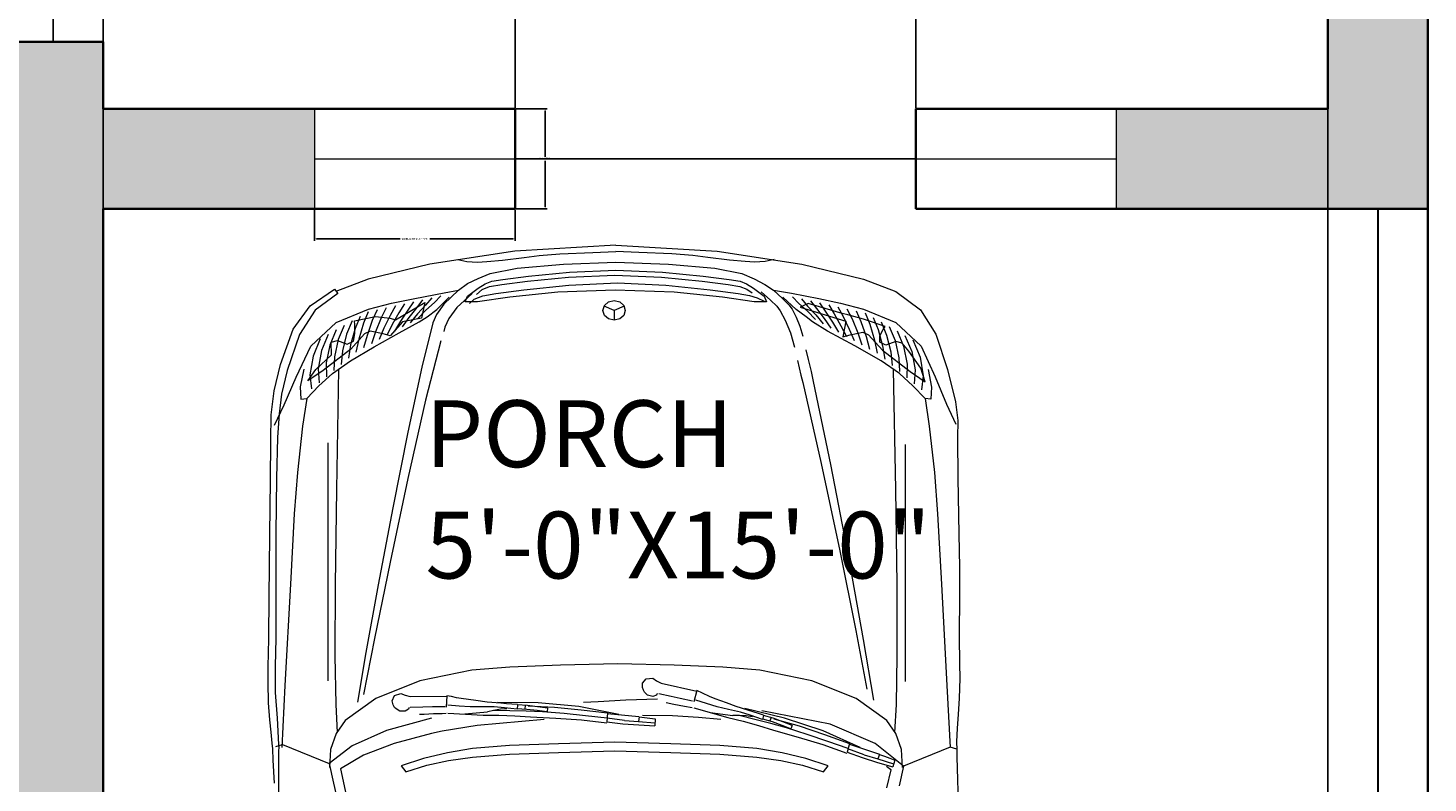
# Model space of a CAD drawing. Units: inches. Extents: x -16 to 587, y -783 to 64.
# Tile 6 of 14: x 111 to 237, y -595 to -527. Entities that reach past the tile are written whole.
import ezdxf

# ---------------------------------------------------------------- set-up
doc = ezdxf.new("R2010")
doc.units = ezdxf.units.IN
doc.header["$MEASUREMENT"] = 0
for name, color, linetype, lineweight in [('A-ANNO-DIMS', 2, 'Continuous', 18), ('A-AREA-IDEN', 7, 'Continuous', 18), ('A-DOOR', 3, 'Continuous', 25), ('A-GLAZ', 4, 'Continuous', 18), ('A-SITE-VEHC', 8, 'Continuous', 13), ('A-SITE-WALL', 7, 'Continuous', 30), ('A-WALL', 7, 'Continuous', 35), ('A-WALL-PATT', 23, 'Continuous', 13)]:
    doc.layers.add(name, color=color, linetype=linetype, lineweight=lineweight)
doc.styles.get("Standard").update_dxf_attribs({"font": 'arial.ttf'})
doc.dimstyles.get("Standard").update_dxf_attribs({"dimtxt": 0.18, "dimasz": 0.18, "dimexe": 0.18, "dimexo": 0.0625, "dimgap": 0.09, "dimtad": 0, "dimtih": 1, "dimtoh": 1, "dimdec": 0, "dimzin": 0, "dimdsep": 46, "dimlunit": 3, "dimtxsty": 'Standard', "dimcen": 0.09, "dimadec": 0, "dimazin": 0, "dimtfac": 1, "dimtdec": 0, "dimtofl": 0, "dimtmove": 0, "dimatfit": 3, "dimfxl": 1, "dimtolj": 1, "dimtzin": 0, "dimarcsym": 0})

# ---------------------------------------------------------------- blocks, each defined once
blk = doc.blocks.new('WIN-18-SIDELIGHT')
for p, q in [((6, 9), (0, 9)), ((0, 9), (0, 0)), ((6, 9), (18, 9)), ((18, 9), (18, 0)), ((0, 4.5), (18, 4.5)), ((0, 0), (6, 0)), ((18, 0), (6, 0))]:
    blk.add_line(p, q)
blk = doc.blocks.new('*D48')
at = {"layer": 'A-ANNO-DIMS', "color": 0, "lineweight": -2, "transparency": 16777216}
for p, q in [((137.08, -543.62), (137.08, -546.43)), ((155.08, -543.62), (155.08, -546.43)), ((137.26, -546.25), (144.75, -546.25)), ((154.9, -546.25), (147.42, -546.25))]:
    blk.add_line(p, q, dxfattribs=at)
at = {"layer": 'A-ANNO-DIMS', "color": 0, "transparency": 16777216}
for points in [[(137.26, -546.22), (137.26, -546.28), (137.08, -546.25)], [(154.9, -546.22), (154.9, -546.28), (155.08, -546.25)]]:
    blk.add_solid(points, dxfattribs=at)
at = {"layer": 'Defpoints', "color": 0, "transparency": 16777216}
for p in [(137.08, -543.55), (155.08, -543.55), (155.08, -546.25)]:
    blk.add_point(p, dxfattribs=at)
at = {"layer": 'A-ANNO-DIMS', "color": 0, "transparency": 16777216, "insert": (146.08, -546.25), "char_height": 0.18, "attachment_point": 5}
blk.add_mtext('\\A1;SIDELIGHT 1\'-6" TYP.', dxfattribs=at)
blk = doc.blocks.new('*D49')
at = {"layer": 'A-ANNO-DIMS', "color": 0, "lineweight": -2, "transparency": 16777216}
for p, q in [((155.15, -534.55), (157.96, -534.55)), ((157.78, -534.73), (157.78, -538.87)), ((157.78, -543.37), (157.78, -539.24)), ((155.15, -543.55), (157.96, -543.55))]:
    blk.add_line(p, q, dxfattribs=at)
at = {"layer": 'A-ANNO-DIMS', "color": 0, "transparency": 16777216}
for points in [[(157.75, -534.73), (157.81, -534.73), (157.78, -534.55)], [(157.75, -543.37), (157.81, -543.37), (157.78, -543.55)]]:
    blk.add_solid(points, dxfattribs=at)
at = {"layer": 'Defpoints', "color": 0, "transparency": 16777216}
for p in [(155.08, -534.55), (157.78, -534.55), (155.08, -543.55)]:
    blk.add_point(p, dxfattribs=at)
at = {"layer": 'A-ANNO-DIMS', "color": 0, "transparency": 16777216, "insert": (157.78, -539.05), "char_height": 0.18, "attachment_point": 5}
blk.add_mtext('\\A1;0\'-9" TYP.', dxfattribs=at)
blk = doc.blocks.new('*D56')
at = {"layer": 'A-ANNO-DIMS', "color": 0, "lineweight": -2, "transparency": 16777216}
for p, q in [((118.08, -728.49), (118.08, 63.78)), ((118.26, 63.6), (172.75, 63.6)), ((227.9, 63.6), (173.41, 63.6)), ((228.08, -728.49), (228.08, 63.78))]:
    blk.add_line(p, q, dxfattribs=at)
at = {"layer": 'A-ANNO-DIMS', "color": 0, "transparency": 16777216}
for points in [[(118.26, 63.63), (118.26, 63.57), (118.08, 63.6)], [(227.9, 63.63), (227.9, 63.57), (228.08, 63.6)]]:
    blk.add_solid(points, dxfattribs=at)
at = {"layer": 'Defpoints', "color": 0, "transparency": 16777216}
for p in [(228.08, 63.6), (118.08, -728.55), (228.08, -728.55)]:
    blk.add_point(p, dxfattribs=at)
at = {"layer": 'A-ANNO-DIMS', "color": 0, "transparency": 16777216, "insert": (173.08, 63.6), "char_height": 0.18, "attachment_point": 5}
blk.add_mtext('\\A1;9\'-2"', dxfattribs=at)
blk = doc.blocks.new('*D57')
at = {"layer": 'A-ANNO-DIMS', "color": 0, "lineweight": -2, "transparency": 16777216}
for p, q in [((155.08, -534.49), (155.08, 63.78)), ((155.26, 63.6), (172.75, 63.6)), ((190.9, 63.6), (173.41, 63.6)), ((191.08, -534.49), (191.08, 63.78))]:
    blk.add_line(p, q, dxfattribs=at)
at = {"layer": 'A-ANNO-DIMS', "color": 0, "transparency": 16777216}
for points in [[(155.26, 63.63), (155.26, 63.57), (155.08, 63.6)], [(190.9, 63.63), (190.9, 63.57), (191.08, 63.6)]]:
    blk.add_solid(points, dxfattribs=at)
at = {"layer": 'Defpoints', "color": 0, "transparency": 16777216}
for p in [(191.08, 63.6), (155.08, -534.55), (191.08, -534.55)]:
    blk.add_point(p, dxfattribs=at)
at = {"layer": 'A-ANNO-DIMS', "color": 0, "transparency": 16777216, "insert": (173.08, 63.6), "char_height": 0.18, "attachment_point": 5}
blk.add_mtext('\\A1;3\'-0"', dxfattribs=at)

msp = doc.modelspace()

# ---------------------------------------------------------------- hatches: boundary and pattern name
at = {"layer": 'A-WALL-PATT'}
h = msp.add_hatch(color=256, dxfattribs=at)
h.dxf.hatch_style = 1
h.paths.add_polyline_path([(137.08, -543.55), (137.08, -534.55), (118.08, -534.55), (118.08, -528.55), (109.08, -528.55), (109.08, -534.55), (109.08, -672.55), (118.08, -672.55), (118.08, -543.55)], flags=17)
h.paths.add_polyline_path([(27.08, -663.55), (27.08, -400.55), (73.08, -400.55), (73.08, -391.55), (27.08, -391.55), (27.08, 10.45), (48.75, 10.45), (171.08, 10.45), (171.08, -17.55), (180.08, -17.55), (180.08, 10.45), (228.08, 10.45), (228.08, -262.55), (206.41, -262.55), (118.08, -262.55), (118.08, -271.55), (228.08, -271.55), (228.08, -391.55), (154.08, -391.55), (154.08, -400.55), (228.08, -400.55), (228.08, -534.55), (209.08, -534.55), (209.08, -543.55), (237.08, -543.55), (237.08, 19.45), (18.08, 19.45), (18.08, -672.55), (73.08, -672.55), (73.08, -663.55)])
h.paths.add_polyline_path([(109.08, -486.55), (87.08, -486.55), (87.08, -495.55), (118.08, -495.55), (118.08, -400.55), (118.08, -391.55), (109.08, -391.55), (109.08, -400.55)], flags=17)

# ---------------------------------------------------------------- linework, layer by layer
at = {"layer": 'A-DOOR'}
for p, q in [((113.58, -528.55), (113.58, -495.55)), ((155.08, -539.05), (191.08, -539.05))]:
    msp.add_line(p, q, dxfattribs=at)
at = {"layer": 'A-SITE-VEHC'}
for p, q in [((164.14, -546.8), (155.05, -547.34)), ((164.14, -546.8), (173.23, -547.34)), ((155.05, -547.34), (147.44, -548.5)), ((149.93, -548.1), (150.74, -548.27)), ((150.74, -548.27), (151.7, -548.32)), ((152.55, -548.28), (153.94, -548.14)), ((153.94, -548.14), (155.9, -547.93)), ((155.9, -547.93), (157.25, -547.75)), ((157.25, -547.75), (159.11, -547.6)), ((159.11, -547.6), (162.08, -547.46)), ((162.08, -547.46), (164.14, -547.39)), ((166.21, -547.46), (164.14, -547.39)), ((169.17, -547.6), (166.21, -547.46)), ((171.04, -547.75), (169.17, -547.6)), ((172.39, -547.93), (171.04, -547.75)), ((174.35, -548.14), (172.39, -547.93)), ((173.23, -547.34), (180.84, -548.5)), ((175.74, -548.28), (174.35, -548.14)), ((177.54, -548.27), (176.59, -548.32)), ((178.35, -548.1), (177.54, -548.27)), ((147.44, -548.5), (141.89, -549.85)), ((151.7, -548.32), (152.55, -548.28)), ((151.77, -549.79), (152.85, -549.35)), ((152.85, -549.35), (155.26, -548.88)), ((155.26, -548.88), (159.43, -548.5)), ((156.29, -549.59), (159.96, -549.23)), ((159.43, -548.5), (164.14, -548.34)), ((159.87, -549.69), (164.05, -549.51)), ((159.96, -549.23), (164.14, -549.06)), ((164.05, -549.51), (168.23, -549.69)), ((164.14, -548.34), (168.85, -548.5)), ((164.14, -549.06), (168.32, -549.23)), ((168.32, -549.23), (171.99, -549.59)), ((168.85, -548.5), (173.03, -548.88)), ((173.03, -548.88), (175.44, -549.35)), ((175.44, -549.35), (176.55, -549.83)), ((176.59, -548.32), (175.74, -548.28)), ((180.84, -548.5), (186.39, -549.85)), ((136.67, -552.25), (138.87, -550.75)), ((138.87, -550.75), (139.16, -551.16)), ((141.89, -549.85), (138.99, -550.96)), ((149.99, -550.84), (150.81, -550.24)), ((150.81, -550.24), (151.77, -549.79)), ((150.82, -551.38), (151.78, -550.66)), ((151.78, -550.66), (152.41, -550.27)), ((152.12, -550.8), (152.8, -550.53)), ((152.41, -550.27), (152.98, -550.05)), ((152.8, -550.53), (153.88, -550.35)), ((152.98, -550.05), (153.98, -549.89)), ((153.88, -550.35), (156.2, -550.05)), ((153.98, -549.89), (156.29, -549.59)), ((155.88, -550.83), (159.9, -550.41)), ((156.2, -550.05), (159.87, -549.69)), ((159.9, -550.41), (164.28, -550.2)), ((164.28, -550.2), (168.63, -550.41)), ((168.23, -549.69), (171.9, -550.05)), ((168.63, -550.41), (172.62, -550.83)), ((171.9, -550.05), (174.22, -550.35)), ((171.99, -549.59), (174.31, -549.89)), ((174.22, -550.35), (175.27, -550.53)), ((174.31, -549.89), (175.31, -550.05)), ((175.27, -550.53), (175.91, -550.75)), ((175.31, -550.05), (175.88, -550.27)), ((175.88, -550.27), (176.51, -550.66)), ((175.91, -550.75), (176.37, -551.09)), ((176.51, -550.66), (177.46, -551.38)), ((176.55, -549.83), (177.53, -550.33)), ((177.53, -550.33), (178.29, -550.84)), ((186.39, -549.85), (189.29, -550.96)), ((139.16, -551.16), (137.13, -552.65)), ((141.91, -552.55), (143.99, -552.03)), ((143.99, -552.03), (146.07, -551.59)), ((144.33, -553.5), (146.99, -551.96)), ((145.96, -551.9), (145.45, -552.65)), ((146.07, -551.59), (148.7, -551.08)), ((146.78, -551.72), (146.25, -552.42)), ((146.99, -551.96), (146.67, -553.37)), ((147.6, -551.54), (147.05, -552.19)), ((147.84, -551.96), (147.06, -552.65)), ((148.41, -551.36), (147.84, -551.96)), ((148.04, -552.58), (149.16, -551.49)), ((149.99, -550.84), (148.67, -552.1)), ((148.7, -551.08), (149.99, -550.84)), ((151.23, -551.15), (149.86, -552.41)), ((150.61, -551.9), (150.82, -551.38)), ((151.72, -551.91), (150.61, -551.9)), ((150.98, -552.05), (151.4, -551.67)), ((151.4, -551.67), (152.19, -551.37)), ((151.62, -551.23), (152.12, -550.8)), ((154.6, -551.47), (151.72, -551.91)), ((152.19, -551.37), (153.36, -551.16)), ((153.36, -551.16), (155.88, -550.83)), ((158.92, -551.04), (154.6, -551.47)), ((164.08, -550.84), (158.92, -551.04)), ((163.1, -552.22), (163.46, -551.9)), ((163.46, -551.9), (163.97, -551.78)), ((163.97, -551.78), (164.48, -551.9)), ((169.38, -551.04), (164.08, -550.84)), ((164.48, -551.9), (164.84, -552.22)), ((173.71, -551.47), (169.38, -551.04)), ((172.62, -550.83), (175.11, -551.16)), ((176.57, -551.91), (173.71, -551.47)), ((175.11, -551.16), (176.13, -551.32)), ((176.13, -551.32), (176.84, -551.53)), ((177.68, -551.9), (176.57, -551.91)), ((176.84, -551.53), (177.45, -551.85)), ((177.19, -551), (178.02, -551.75)), ((177.46, -551.38), (177.68, -551.9)), ((178.02, -551.75), (178.58, -552.29)), ((178.29, -550.84), (179.11, -551.6)), ((178.29, -550.84), (179.92, -551.13)), ((179.11, -551.6), (179.66, -552.16)), ((180.32, -552.58), (179.13, -551.49)), ((179.92, -551.13), (182.38, -551.61)), ((179.99, -551.45), (180.56, -552.05)), ((180.81, -551.63), (181.36, -552.28)), ((181.63, -551.81), (182.16, -552.51)), ((182.38, -551.61), (184.3, -552.03)), ((182.44, -551.99), (182.95, -552.74)), ((184.3, -552.03), (186.38, -552.55)), ((189.29, -550.96), (191.51, -552.62)), ((135.15, -554.34), (136.67, -552.25)), ((137.13, -552.65), (135.73, -554.84)), ((139.01, -553.74), (141.91, -552.55)), ((140.67, -553.6), (142.56, -553.21)), ((141.16, -553.2), (140.71, -554.29)), ((141.88, -552.8), (141.46, -553.8)), ((142.69, -552.62), (142.26, -553.57)), ((142.56, -553.21), (143.85, -553.35)), ((143.51, -552.44), (143.06, -553.34)), ((143.85, -553.11), (143.3, -554.27)), ((144.33, -552.26), (143.85, -553.11)), ((144.65, -552.88), (144.05, -553.94)), ((145.14, -552.08), (144.65, -552.88)), ((145.45, -552.65), (144.8, -553.62)), ((145.55, -553.3), (144.95, -554.15)), ((146.25, -552.42), (145.55, -553.3)), ((146.31, -552.97), (145.65, -553.78)), ((147.05, -552.19), (146.31, -552.97)), ((147.06, -552.65), (146.34, -553.4)), ((146.48, -553.69), (147.2, -553.25)), ((147.2, -553.25), (148.04, -552.58)), ((148.01, -553.02), (147.71, -553.77)), ((148.67, -552.1), (148.01, -553.02)), ((149.86, -552.41), (149.12, -553.4)), ((162.97, -552.67), (163.1, -552.22)), ((163.1, -553.11), (162.97, -552.67)), ((163.97, -552.67), (163.07, -552.28)), ((163.46, -553.43), (163.1, -553.11)), ((164.87, -552.28), (163.97, -552.67)), ((163.97, -552.67), (163.97, -553.55)), ((164.84, -553.11), (164.48, -553.43)), ((164.84, -552.22), (164.97, -552.67)), ((164.97, -552.67), (164.84, -553.11)), ((178.58, -552.29), (178.89, -552.7)), ((178.89, -552.7), (179.35, -553.55)), ((179.66, -552.16), (179.96, -552.56)), ((179.96, -552.56), (180.34, -553.28)), ((181.24, -553.24), (180.32, -552.58)), ((180.34, -553.28), (180.66, -554.09)), ((180.56, -552.05), (181.35, -552.74)), ((181.41, -552.05), (180.69, -552.37)), ((180.69, -552.37), (184.8, -553.64)), ((181.8, -553.69), (181.24, -553.24)), ((181.35, -552.74), (182.06, -553.49)), ((181.36, -552.28), (182.1, -553.07)), ((184.45, -552.94), (181.41, -552.05)), ((182.1, -553.07), (182.75, -553.87)), ((182.16, -552.51), (182.85, -553.39)), ((182.95, -552.74), (183.6, -553.71)), ((183.26, -552.17), (183.75, -552.97)), ((183.75, -552.97), (184.35, -554.04)), ((184.08, -552.35), (184.55, -553.2)), ((184.98, -553.07), (184.45, -552.94)), ((184.55, -553.2), (185.1, -554.36)), ((184.89, -552.53), (185.35, -553.43)), ((186.37, -553.46), (184.98, -553.07)), ((185.71, -552.71), (186.15, -553.66)), ((186.38, -552.55), (189.27, -553.74)), ((186.53, -552.89), (186.94, -553.89)), ((187.24, -553.3), (187.7, -554.39)), ((191.51, -552.62), (192.88, -554.79)), ((134, -557.52), (135.15, -554.34)), ((136.73, -555.89), (139.01, -553.74)), ((139.01, -554.42), (138.44, -555.78)), ((139.73, -554.01), (139.2, -555.29)), ((140.45, -553.61), (139.95, -554.79)), ((140.71, -554.29), (140.31, -555.77)), ((140.69, -553.96), (140.67, -553.6)), ((140.7, -554.73), (140.69, -553.96)), ((141.46, -553.8), (141.04, -555.24)), ((142.08, -554.54), (141.56, -554.78)), ((142.26, -553.57), (141.8, -554.91)), ((143.23, -554.76), (142.08, -554.54)), ((143.06, -553.34), (142.55, -554.59)), ((143.3, -554.27), (142.87, -555.29)), ((144.05, -553.94), (143.57, -554.91)), ((143.85, -553.35), (144.33, -553.5)), ((144.97, -553.69), (143.87, -554.94)), ((144.8, -553.62), (144.26, -554.53)), ((144.67, -554.69), (146.48, -553.69)), ((146.67, -553.37), (144.97, -553.69)), ((147.71, -553.77), (146.71, -557.77)), ((148.78, -554.18), (148.67, -554.55)), ((149.12, -553.4), (148.78, -554.18)), ((163.97, -553.55), (163.46, -553.43)), ((164.48, -553.43), (163.97, -553.55)), ((179.35, -553.55), (179.82, -554.69)), ((180.66, -554.09), (180.94, -554.99)), ((183.14, -554.52), (181.8, -553.69)), ((182.85, -553.39), (183.45, -554.25)), ((185.61, -555.86), (183.14, -554.52)), ((183.6, -553.71), (184.14, -554.62)), ((184.35, -554.04), (184.84, -555)), ((184.8, -553.64), (184.53, -555.04)), ((185.1, -554.36), (185.53, -555.38)), ((185.35, -553.43), (185.86, -554.68)), ((186.15, -553.66), (186.61, -555)), ((188.32, -554.12), (186.37, -553.46)), ((186.94, -553.89), (187.36, -555.33)), ((187.7, -554.39), (188.09, -555.86)), ((187.86, -554.94), (188.14, -554.37)), ((187.96, -553.7), (188.45, -554.88)), ((188.14, -554.37), (188.32, -554.12)), ((188.67, -554.1), (189.21, -555.38)), ((189.27, -553.74), (191.55, -555.89)), ((189.39, -554.51), (189.96, -555.87)), ((135.73, -554.84), (134.62, -558.05)), ((137.58, -555.22), (136.94, -556.77)), ((138.3, -554.82), (137.69, -556.28)), ((138.44, -555.78), (138.12, -557.38)), ((138.56, -555.51), (139.13, -555.37)), ((138.6, -556.67), (138.56, -555.51)), ((139.2, -555.29), (138.85, -556.85)), ((139.13, -555.37), (140.01, -555.71)), ((139.95, -554.79), (139.58, -556.31)), ((140.01, -555.71), (140.57, -555.43)), ((140.31, -555.77), (140.13, -556.97)), ((141.56, -554.78), (140.33, -556.16)), ((140.57, -555.43), (140.7, -554.73)), ((141.04, -555.24), (140.79, -556.42)), ((141.8, -554.91), (141.48, -556.04)), ((142.55, -554.59), (142.18, -555.67)), ((142.43, -555.94), (144.67, -554.69)), ((143.87, -554.94), (143.23, -554.76)), ((148.41, -555.4), (147.04, -560.74)), ((179.82, -554.69), (180.19, -555.97)), ((184.53, -555.04), (185.17, -554.85)), ((185.17, -554.85), (186.32, -554.63)), ((185.86, -554.68), (186.23, -555.76)), ((186.32, -554.63), (186.84, -554.87)), ((186.61, -555), (186.92, -556.14)), ((186.84, -554.87), (188.08, -556.25)), ((187.36, -555.33), (187.61, -556.51)), ((187.84, -555.52), (187.86, -554.94)), ((188.39, -555.8), (187.84, -555.52)), ((189.28, -555.46), (188.39, -555.8)), ((188.45, -554.88), (188.82, -556.4)), ((189.21, -555.38), (189.55, -556.94)), ((189.85, -555.6), (189.28, -555.46)), ((190.46, -556.34), (189.85, -555.6)), ((190.1, -554.91), (190.71, -556.37)), ((190.82, -555.31), (191.47, -556.86)), ((192.88, -554.79), (193.93, -557.97)), ((135.41, -558.65), (136.73, -555.89)), ((136.94, -556.77), (136.65, -558.46)), ((137.2, -557.97), (138.6, -556.67)), ((137.69, -556.28), (137.39, -557.92)), ((140.33, -556.16), (137.84, -558.05)), ((138.85, -556.85), (138.8, -558.07)), ((139.58, -556.31), (139.47, -557.52)), ((140.3, -557.2), (142.43, -555.94)), ((181.2, -556.2), (181.41, -557.08)), ((187.98, -557.2), (185.61, -555.86)), ((188.08, -556.25), (190.57, -558.14)), ((188.09, -555.86), (188.28, -557.06)), ((188.82, -556.4), (188.94, -557.61)), ((189.55, -556.94), (189.6, -558.16)), ((189.96, -555.87), (190.29, -557.48)), ((191.53, -557.84), (190.46, -556.34)), ((190.71, -556.37), (191.02, -558.01)), ((191.47, -556.86), (191.75, -558.55)), ((191.55, -555.89), (192.83, -558.63)), ((133.43, -559.88), (134, -557.52)), ((134.62, -558.05), (134.11, -560.18)), ((136.11, -557.93), (135.79, -559.53)), ((136.48, -559), (137.2, -557.97)), ((137.84, -558.05), (136.48, -559)), ((137.39, -557.92), (137.48, -559.17)), ((138.12, -557.38), (138.14, -558.62)), ((138.69, -558.34), (140.3, -557.2)), ((139.23, -557.97), (139.03, -568.74)), ((146.71, -557.77), (145.45, -563.61)), ((180.46, -557.18), (180.61, -557.83)), ((180.61, -557.83), (180.76, -558.49)), ((181.41, -557.08), (181.67, -558.16)), ((181.67, -558.16), (181.87, -559.04)), ((189.6, -558.34), (187.98, -557.2)), ((189.05, -557.97), (189.26, -568.74)), ((190.29, -557.48), (190.26, -558.71)), ((190.57, -558.14), (191.92, -559.09)), ((191.02, -558.01), (190.93, -559.26)), ((191.92, -559.09), (191.53, -557.84)), ((192.19, -557.98), (192.5, -559.56)), ((193.93, -557.97), (194.65, -560.87)), ((134.35, -561.16), (135.41, -558.65)), ((135.79, -559.53), (135.84, -560.64)), ((136.38, -560.59), (137.47, -559.45)), ((136.65, -558.46), (136.81, -559.72)), ((137.47, -559.45), (138.69, -558.34)), ((180.76, -558.49), (180.92, -559.14)), ((180.92, -559.14), (182.58, -566.42)), ((181.87, -559.04), (183.42, -566.51)), ((190.81, -559.45), (189.6, -558.34)), ((191.91, -560.59), (190.81, -559.45)), ((191.75, -558.55), (191.59, -559.81)), ((192.5, -559.56), (192.44, -560.65)), ((192.83, -558.63), (193.82, -561.08)), ((133.16, -562.03), (133.43, -559.88)), ((134.11, -560.18), (133.88, -561.96)), ((135.84, -560.64), (136.38, -560.59)), ((136.38, -560.59), (136, -563.05)), ((147.04, -560.74), (145.45, -567.75)), ((191.91, -560.59), (192.28, -563.05)), ((192.44, -560.65), (191.91, -560.59)), ((133.13, -564.39), (133.16, -562.03)), ((133.46, -562.97), (134.35, -561.16)), ((133.88, -561.96), (133.74, -564.09)), ((193.82, -561.08), (194.67, -562.87)), ((194.65, -560.87), (194.85, -562.55)), ((136, -563.05), (135.54, -567.21)), ((192.28, -563.05), (192.75, -567.21)), ((194.85, -562.55), (194.82, -564.1)), ((133.12, -567.94), (133.13, -564.39)), ((133.74, -564.09), (133.65, -567.72)), ((138.29, -585.93), (138.29, -564.56)), ((145.45, -563.61), (144.1, -570.41)), ((194.82, -564.1), (194.84, -567.73)), ((190.14, -586), (190.14, -564.71)), ((182.58, -566.42), (184.24, -574.26)), ((183.42, -566.51), (184.99, -574.7)), ((133.05, -572.79), (133.12, -567.94)), ((133.65, -567.72), (133.6, -572.71)), ((135.54, -567.21), (135.25, -570.94)), ((145.45, -567.75), (143.86, -575.27)), ((192.75, -567.21), (193.04, -570.94)), ((194.84, -567.73), (194.94, -572.72)), ((139.03, -568.74), (138.92, -577.27)), ((189.26, -568.74), (189.36, -577.27)), ((144.1, -570.41), (142.79, -577.3)), ((135.25, -570.94), (134.91, -577.25)), ((193.04, -570.94), (193.37, -577.25)), ((133.01, -575.75), (133.05, -572.79)), ((133.6, -572.71), (133.58, -575.75)), ((194.94, -572.72), (195, -575.75)), ((184.24, -574.26), (185.69, -581.42)), ((133, -578.29), (133.01, -575.75)), ((133.58, -575.75), (133.58, -578.28)), ((143.86, -575.27), (142.46, -582.12)), ((184.99, -574.7), (186.34, -582.23)), ((195, -575.75), (194.99, -578.21)), ((132.97, -582.17), (133, -578.29)), ((133.58, -578.28), (133.58, -582.14)), ((134.91, -577.25), (134.41, -586.36)), ((138.92, -577.27), (138.9, -583.68)), ((142.79, -577.3), (141.68, -583.4)), ((189.36, -577.27), (189.38, -583.68)), ((193.37, -577.25), (193.87, -586.36)), ((194.99, -578.21), (194.97, -581.95)), ((132.91, -584.67), (132.97, -582.17)), ((133.58, -582.14), (133.54, -584.63)), ((142.46, -582.12), (141.46, -587.15)), ((185.69, -581.42), (186.69, -586.69)), ((194.97, -581.95), (195, -584.37)), ((141.68, -583.4), (140.93, -587.85)), ((186.34, -582.23), (187.27, -587.67)), ((132.89, -586.07), (132.91, -584.67)), ((133.54, -584.63), (133.54, -586.99)), ((138.9, -583.68), (138.97, -588.07)), ((154.62, -584.7), (151.21, -584.97)), ((159.17, -584.53), (154.62, -584.7)), ((164.31, -584.4), (159.17, -584.53)), ((169.36, -584.53), (164.31, -584.4)), ((173.75, -584.7), (169.36, -584.53)), ((177.07, -584.97), (173.75, -584.7)), ((189.38, -583.68), (189.32, -588.07)), ((195, -584.37), (195.02, -585.72)), ((146.53, -585.94), (142.58, -587.52)), ((151.21, -584.97), (146.53, -585.94)), ((166.54, -586.15), (166.85, -585.75)), ((166.85, -585.75), (167.45, -585.69)), ((167.45, -585.69), (167.79, -585.92)), ((167.79, -585.92), (168.2, -586.14)), ((181.75, -585.94), (177.07, -584.97)), ((185.71, -587.52), (181.75, -585.94)), ((195.02, -585.72), (194.98, -587.49)), ((132.94, -587.92), (132.89, -586.07)), ((133.54, -586.99), (133.72, -589.29)), ((134.41, -586.36), (134.12, -591.92)), ((144.26, -587.26), (144.83, -587.06)), ((144.83, -587.06), (145.22, -587.22)), ((145.22, -587.22), (145.67, -587.34)), ((166.53, -586.53), (166.54, -586.15)), ((166.61, -586.78), (166.53, -586.53)), ((166.7, -586.94), (166.61, -586.78)), ((166.98, -587.23), (166.7, -586.94)), ((167.45, -587.33), (166.98, -587.23)), ((167.78, -587.22), (167.45, -587.33)), ((167.83, -587.12), (167.78, -587.22)), ((167.89, -587.08), (167.83, -587.12)), ((169.09, -587.33), (167.98, -587.1)), ((168.2, -586.14), (171.4, -586.86)), ((171.42, -586.81), (171.13, -587.81)), ((171.92, -587.04), (171.42, -586.81)), ((172.54, -587.35), (171.92, -587.04)), ((193.87, -586.36), (194.17, -591.92)), ((133.04, -589.43), (132.94, -587.92)), ((138.97, -588.07), (139.11, -590.56)), ((142.58, -587.52), (139.82, -589.49)), ((144.05, -587.72), (144.26, -587.26)), ((144.13, -588.09), (144.05, -587.72)), ((144.26, -588.32), (144.13, -588.09)), ((144.39, -588.46), (144.26, -588.32)), ((144.73, -588.67), (144.39, -588.46)), ((145.5, -588.49), (145.21, -588.66)), ((145.53, -588.38), (145.5, -588.49)), ((145.58, -588.32), (145.53, -588.38)), ((145.67, -587.34), (148.95, -587.32)), ((146.81, -588.3), (145.67, -588.32)), ((147.66, -588.28), (146.81, -588.3)), ((148.79, -588.27), (147.66, -588.28)), ((148.96, -587.27), (148.9, -588.31)), ((149.38, -587.35), (148.96, -587.27)), ((150.07, -588.2), (149.04, -588.13)), ((149.82, -587.46), (149.38, -587.35)), ((150.25, -587.53), (149.82, -587.46)), ((151.06, -588.26), (150.07, -588.2)), ((151.57, -587.71), (150.25, -587.53)), ((152.08, -588.27), (151.06, -588.26)), ((152.57, -587.85), (151.57, -587.71)), ((153.21, -588.27), (152.08, -588.27)), ((153.81, -587.95), (152.57, -587.85)), ((153.76, -588.48), (153.18, -588.6)), ((154.12, -588.35), (153.21, -588.27)), ((157.17, -587.91), (153.51, -587.88)), ((154.35, -588.44), (153.76, -588.48)), ((154.3, -587.99), (153.81, -587.95)), ((155.27, -588.47), (154.12, -588.35)), ((154.8, -588.03), (154.3, -587.99)), ((155.29, -588.07), (154.8, -588.03)), ((155.25, -588.41), (156.15, -588.47)), ((155.3, -588.1), (155.27, -588.47)), ((156.19, -588.15), (155.28, -588.09)), ((155.98, -588.14), (155.95, -588.45)), ((156.15, -588.47), (157.06, -588.57)), ((157.1, -588.26), (156.19, -588.15)), ((156.25, -588.18), (158.63, -588.29)), ((158, -588.39), (157.1, -588.26)), ((160.81, -588.23), (157.17, -587.91)), ((158, -588.39), (157.95, -588.7)), ((158.63, -588.29), (161.01, -588.54)), ((164.4, -588.96), (160.81, -588.23)), ((162.55, -587.81), (161.24, -587.88)), ((165.02, -587.67), (162.55, -587.81)), ((167.89, -587.59), (165.02, -587.67)), ((168.64, -587.87), (169.34, -588.03)), ((169.92, -587.51), (169.09, -587.33)), ((169.34, -588.03), (170.31, -588.21)), ((171.03, -587.75), (169.92, -587.51)), ((170.31, -588.21), (171, -588.33)), ((171.15, -588.35), (174.2, -589.24)), ((172.29, -587.97), (171.31, -587.67)), ((173.24, -588.26), (172.29, -587.97)), ((173.05, -587.56), (172.54, -587.35)), ((174.07, -587.9), (173.05, -587.56)), ((174.24, -588.5), (173.24, -588.26)), ((174.95, -588.24), (174.07, -587.9)), ((175.34, -588.75), (174.24, -588.5)), ((175.99, -588.57), (174.95, -588.24)), ((179.28, -589.29), (175.72, -588.43)), ((188.46, -589.49), (185.71, -587.52)), ((189.32, -588.07), (189.17, -590.56)), ((194.98, -587.49), (194.88, -588.95)), ((133.16, -590.55), (133.04, -589.43)), ((133.72, -589.29), (133.82, -591.65)), ((139.82, -589.49), (139, -590.67)), ((147.59, -589.28), (143.54, -590.4)), ((145.21, -588.66), (144.73, -588.67)), ((146.49, -588.92), (146.91, -588.93)), ((146.91, -588.93), (147.34, -588.91)), ((147.34, -588.91), (147.77, -588.88)), ((147.77, -588.88), (148.14, -588.87)), ((148.14, -588.87), (148.52, -588.86)), ((148.52, -588.86), (148.89, -588.84)), ((149.04, -588.83), (152.21, -589.01)), ((150.56, -588.91), (152.61, -588.71)), ((157.69, -589.4), (151.69, -589.95)), ((152.21, -589.01), (153.62, -589.02)), ((153.18, -588.6), (152.61, -588.71)), ((154.62, -588.64), (153.15, -588.6)), ((153.62, -589.02), (155.05, -589.09)), ((156.09, -588.66), (154.62, -588.64)), ((155.05, -589.09), (156.46, -589.18)), ((157.56, -588.72), (156.09, -588.66)), ((156.46, -589.18), (158.74, -589.29)), ((157.06, -588.57), (157.96, -588.69)), ((159.49, -588.88), (157.56, -588.72)), ((158.74, -589.29), (161.06, -589.45)), ((161.42, -589.09), (159.49, -588.88)), ((161.01, -588.54), (163.38, -588.8)), ((161.06, -589.45), (163.33, -589.7)), ((163.36, -589.28), (161.42, -589.09)), ((163.38, -588.8), (163.33, -589.63)), ((163.33, -589.63), (164.77, -589.79)), ((164.9, -589.5), (163.34, -589.3)), ((163.38, -588.87), (164.32, -588.96)), ((164.32, -588.96), (165.27, -589.05)), ((164.9, -589.5), (166.18, -589.6)), ((165.27, -589.05), (166.21, -589.14)), ((166.22, -589.17), (166.18, -589.6)), ((166.18, -589.6), (167.65, -589.7)), ((166.22, -589.17), (166.7, -589.23)), ((169.22, -589.09), (166.54, -589.05)), ((166.7, -589.23), (167.19, -589.29)), ((167.19, -589.29), (167.67, -589.35)), ((167.67, -589.35), (167.64, -589.98)), ((171.57, -589.23), (169.22, -589.09)), ((173.57, -589.42), (171.57, -589.23)), ((172.61, -588.77), (174.65, -589.04)), ((174.2, -589.24), (175.57, -589.57)), ((175.24, -589.06), (174.65, -589.04)), ((176.62, -589.42), (175.2, -589.05)), ((175.83, -589.08), (175.24, -589.06)), ((176.21, -589.03), (175.34, -588.75)), ((175.57, -589.57), (176.94, -589.96)), ((176.41, -589.17), (175.83, -589.08)), ((176.46, -588.71), (175.99, -588.57)), ((177.3, -589.41), (176.21, -589.03)), ((176.94, -588.87), (176.46, -588.71)), ((178.05, -589.77), (176.62, -589.42)), ((177.41, -589.02), (176.94, -588.87)), ((183.37, -589.82), (177.26, -588.63)), ((177.41, -589.05), (177.3, -589.41)), ((177.3, -589.34), (178.16, -589.6)), ((178.27, -589.3), (177.4, -589.04)), ((178.07, -589.24), (177.96, -589.54)), ((178.16, -589.6), (179.03, -589.91)), ((179.13, -589.61), (178.27, -589.3)), ((178.32, -589.34), (180.61, -589.98)), ((179.97, -589.94), (179.13, -589.61)), ((182.76, -590.42), (179.28, -589.29)), ((189.29, -590.67), (188.46, -589.49)), ((194.88, -588.95), (194.78, -590.19)), ((133.26, -591.53), (133.16, -590.55)), ((139, -590.67), (138.51, -592.1)), ((143.54, -590.4), (140.46, -591.78)), ((147.59, -590.66), (144.21, -591.55)), ((148.52, -590.44), (147.59, -590.66)), ((151.69, -589.95), (148.52, -590.44)), ((164.77, -589.79), (166.2, -589.9)), ((166.2, -589.9), (167.64, -589.98)), ((176.94, -589.96), (178.3, -590.36)), ((179.47, -590.16), (178.05, -589.77)), ((178.3, -590.36), (180.5, -590.99)), ((179.03, -589.91), (179.87, -590.23)), ((181.32, -590.75), (179.47, -590.16)), ((179.97, -589.94), (179.86, -590.23)), ((180.5, -590.99), (182.72, -591.66)), ((180.61, -589.98), (182.88, -590.76)), ((183.16, -591.39), (181.32, -590.75)), ((186.08, -591.93), (182.76, -590.42)), ((182.88, -590.76), (185.13, -591.55)), ((187.42, -591.57), (183.37, -589.82)), ((189.78, -592.1), (189.29, -590.67)), ((194.78, -590.19), (194.74, -591.42)), ((133.31, -592.05), (133.26, -591.53)), ((133.36, -593.07), (133.31, -592.05)), ((133.58, -591.82), (134.18, -591.64)), ((133.82, -591.65), (133.84, -591.69)), ((133.84, -591.69), (133.85, -591.75)), ((133.86, -591.81), (133.84, -592.34)), ((133.85, -591.75), (133.86, -591.81)), ((134.18, -591.64), (138.37, -593.35)), ((140.46, -591.78), (138.37, -593.35)), ((138.51, -592.1), (138.4, -593.71)), ((144.21, -591.55), (141.48, -592.62)), ((151.26, -592.02), (149.01, -592.39)), ((154.59, -591.75), (151.26, -592.02)), ((158.98, -591.58), (154.59, -591.75)), ((164.03, -591.45), (158.98, -591.58)), ((158.98, -592.36), (164.03, -592.23)), ((169.08, -591.58), (164.03, -591.45)), ((164.03, -592.23), (169.08, -592.36)), ((173.48, -591.75), (169.08, -591.58)), ((176.8, -592.02), (173.48, -591.75)), ((179.06, -592.39), (176.8, -592.02)), ((182.72, -591.66), (184.88, -592.42)), ((185, -592.02), (183.16, -591.39)), ((185.13, -591.55), (184.9, -592.35)), ((186.45, -592.57), (184.98, -592.03)), ((185.11, -591.62), (186.01, -591.92)), ((186.01, -591.92), (186.91, -592.21)), ((186.91, -592.21), (187.81, -592.52)), ((189.97, -593.61), (187.42, -591.57)), ((189.89, -593.71), (189.78, -592.1)), ((194.17, -591.89), (189.97, -593.61)), ((194.76, -592.07), (194.17, -591.89)), ((194.74, -591.42), (194.76, -592.1)), ((194.76, -592.1), (194.77, -592.75)), ((133.46, -595.13), (133.36, -593.07)), ((133.84, -592.34), (133.83, -594.2)), ((138.37, -593.35), (138.78, -595.11)), ((141.48, -592.62), (139.4, -593.83)), ((146.85, -592.91), (144.85, -593.58)), ((145.26, -594.11), (147.15, -593.51)), ((149.01, -592.39), (146.85, -592.91)), ((147.15, -593.51), (149.11, -593.1)), ((149.11, -593.1), (151.26, -592.8)), ((151.26, -592.8), (154.59, -592.53)), ((154.59, -592.53), (158.98, -592.36)), ((169.08, -592.36), (173.48, -592.53)), ((173.48, -592.53), (176.8, -592.8)), ((176.8, -592.8), (178.95, -593.1)), ((178.95, -593.1), (180.91, -593.51)), ((181.21, -592.91), (179.06, -592.39)), ((180.91, -593.51), (182.8, -594.11)), ((183.21, -593.58), (181.21, -592.91)), ((184.9, -592.35), (186.26, -592.83)), ((186.26, -592.83), (187.63, -593.26)), ((186.45, -592.57), (187.68, -592.95)), ((187.63, -593.26), (189.01, -593.66)), ((187.81, -592.55), (187.68, -592.95)), ((187.68, -592.95), (189.08, -593.39)), ((187.81, -592.55), (188.27, -592.71)), ((188.27, -592.71), (188.73, -592.88)), ((188.73, -592.88), (189.18, -593.06)), ((189.18, -593.06), (189.01, -593.66)), ((194.77, -592.75), (194.82, -594.81)), ((133.83, -594.2), (133.86, -597.86)), ((139.4, -593.83), (143.12, -610.83)), ((144.85, -593.58), (145.26, -594.11)), ((182.8, -594.11), (183.21, -593.58)), ((188.57, -593.73), (188.43, -593.64)), ((188.47, -595.54), (188.85, -593.94)), ((188.71, -593.83), (188.57, -593.73)), ((188.85, -593.94), (188.71, -593.83)), ((189.97, -593.61), (189.57, -595.36)), ((138.78, -595.11), (139.64, -598.89)), ((194.82, -594.81), (194.93, -598.46))]:
    msp.add_line(p, q, dxfattribs=at)
at = {"layer": 'A-SITE-WALL'}
msp.add_line((232.58, -543.55), (232.58, -728.55), dxfattribs=at)
at = {"layer": 'A-WALL'}
for p, q in [((237.08, 19.45), (237.08, -737.55)), ((228.08, -400.55), (228.08, -534.55)), ((118.08, -528.55), (109.08, -528.55)), ((118.08, -534.55), (118.08, -528.55)), ((118.08, -534.55), (155.08, -534.55)), ((155.08, -543.55), (155.08, -534.55)), ((155.08, -534.55), (155.08, -534.55)), ((191.08, -543.55), (191.08, -534.55)), ((191.08, -534.55), (191.08, -543.55)), ((191.08, -534.55), (228.08, -534.55)), ((118.08, -543.55), (155.08, -543.55)), ((118.08, -543.55), (118.08, -672.55)), ((191.08, -543.55), (237.08, -543.55))]:
    msp.add_line(p, q, dxfattribs=at)

# ---------------------------------------------------------------- block references
at = {"layer": 'A-GLAZ'}
for p in [(137.08, -543.55), (191.08, -543.55)]:
    msp.add_blockref('WIN-18-SIDELIGHT', p, dxfattribs=at)

# ---------------------------------------------------------------- texts
at = {"layer": 'A-AREA-IDEN', "insert": (147.04, -560.74), "char_height": 6, "attachment_point": 1}
msp.add_mtext('PORCH\\P5\'-0"X15\'-0"', dxfattribs=at)

# ---------------------------------------------------------------- dimensions: what is measured, and where the dimension line sits
at = {"layer": 'A-ANNO-DIMS'}
for base, p1, p2, picture in [((228.08, 63.6), (118.08, -728.55), (228.08, -728.55), '*D56'), ((191.08, 63.6), (155.08, -534.55), (191.08, -534.55), '*D57')]:
    dim = msp.add_linear_dim(base=base, p1=p1, p2=p2, dimstyle='Standard', override={"dimdec": 1, "dimlfac": 1, "dimrnd": 0, "dimzin": 1, "dimdsep": 46, "dimlunit": 4, "dimfrac": 2}, dxfattribs=at)
    dim.commit()
    dim.dimension.update_dxf_attribs({"geometry": picture, "text_midpoint": (173.08, 63.6)})
dim = msp.add_linear_dim(base=(157.78, -534.55), p1=(155.08, -543.55), p2=(155.08, -534.55), angle=90, text='<> TYP.', dimstyle='Standard', override={"dimdec": 1, "dimlfac": 1, "dimrnd": 0, "dimzin": 1, "dimdsep": 46, "dimlunit": 4, "dimfrac": 2}, dxfattribs=at)
dim.commit()
dim.dimension.update_dxf_attribs({"geometry": '*D49', "text_midpoint": (157.78, -539.05)})
dim = msp.add_linear_dim(base=(155.08, -546.25), p1=(137.08, -543.55), p2=(155.08, -543.55), text='SIDELIGHT <> TYP.', dimstyle='Standard', override={"dimdec": 1, "dimlfac": 1, "dimrnd": 0, "dimzin": 1, "dimdsep": 46, "dimlunit": 4, "dimfrac": 2}, dxfattribs=at)
dim.commit()
dim.dimension.update_dxf_attribs({"geometry": '*D48', "text_midpoint": (146.08, -546.25)})

doc.saveas('drawing.dxf')
